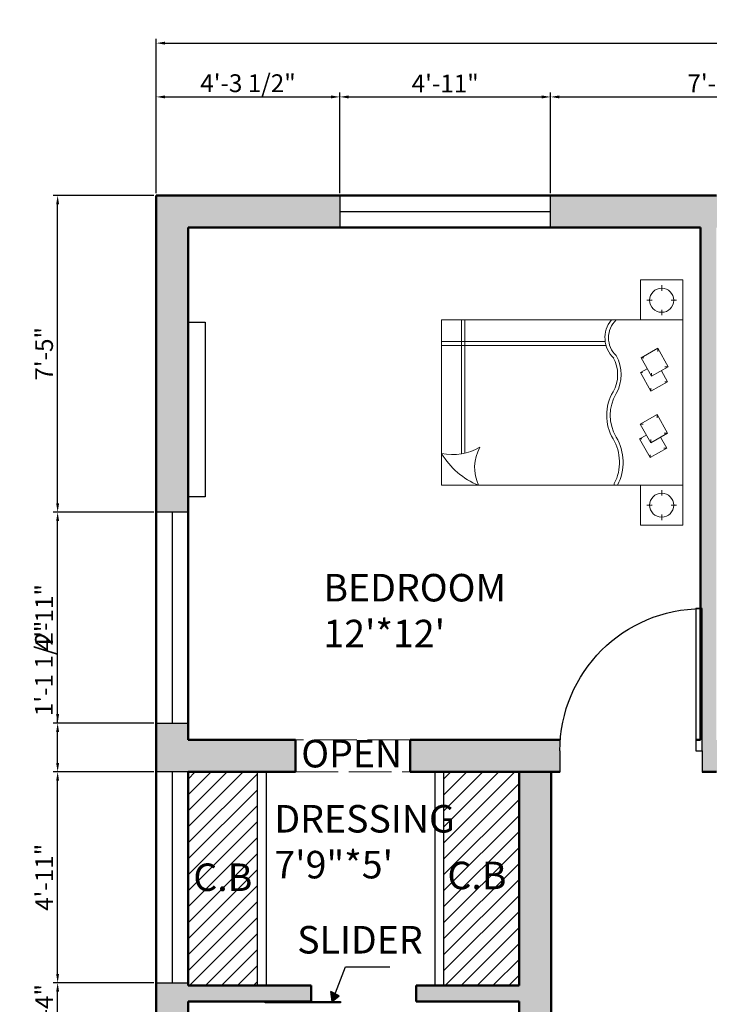
# Model space of a CAD drawing. Units: inches. Extents: x 876 to 1414, y 2665 to 3216.
# Tile 3 of 4: x 876 to 1070, y 2939 to 3216. Entities that reach past the tile are written whole.
import ezdxf

# ---------------------------------------------------------------- set-up
doc = ezdxf.new("R2010")
doc.units = ezdxf.units.IN
doc.linetypes.add('ACAD_ISO02W100', pattern=[15, 12, -3])
for name, color, linetype, lineweight in [('A-ANNO-DIMS', 2, 'Continuous', 18), ('A-ANNO-TEXT', 7, 'Continuous', 25), ('A-AREA-IDEN', 7, 'Continuous', 25), ('A-FLOR-CASE', 8, 'Continuous', 25), ('A-FLOR-CASE-PATT', 252, 'Continuous', 13), ('A-OPEN-OVHD', 210, 'ACAD_ISO02W100', 18), ('A-WALL-PATT', 252, 'Continuous', 13), ('DOOR', 52, 'Continuous', 25), ('FUR', 8, 'Continuous', 18), ('WALL', 7, 'Continuous', 50), ('WIND', 130, 'Continuous', 25)]:
    doc.layers.add(name, color=color, linetype=linetype, lineweight=lineweight)
doc.styles.get("Standard").update_dxf_attribs({"font": 'arial.ttf'})
doc.dimstyles.new('ISO-25', dxfattribs={"dimtxt": 5, "dimasz": 2.5, "dimexe": 1.25, "dimexo": 0.625, "dimtad": 1, "dimdec": 0, "dimlunit": 4, "dimtxsty": 'Standard', "dimcen": 2.5, "dimadec": 0, "dimazin": 0, "dimtfac": 1, "dimtdec": 0, "dimtmove": 0, "dimatfit": 3, "dimfxl": 1, "dimarcsym": 0})

# ---------------------------------------------------------------- blocks, each defined once
blk = doc.blocks.new('*U2')
for p, q in [((0, 0), (0, -6)), ((40, 0), (40, -6))]:
    blk.add_line(p, q)
blk.add_lwpolyline([(0, 0), (0, 40), (1.75, 40), (1.75, 0)], close=True)
blk.add_arc((0, 0), 40, 0, 90)
blk = doc.blocks.new('*D7')
at = {"layer": 'A-ANNO-DIMS', "color": 0, "lineweight": -2, "transparency": 16777216}
for p, q in [((914.52, 3167.07), (914.52, 3210.51)), ((1361.52, 3167.07), (1361.52, 3210.51)), ((917.02, 3209.26), (1359.02, 3209.26))]:
    blk.add_line(p, q, dxfattribs=at)
at = {"layer": 'A-ANNO-DIMS', "color": 0, "lineweight": 100, "transparency": 16777216}
for points in [[(917.02, 3209.68), (917.02, 3208.84), (914.52, 3209.26)], [(1359.02, 3209.68), (1359.02, 3208.84), (1361.52, 3209.26)]]:
    blk.add_solid(points, dxfattribs=at)
at = {"layer": 'Defpoints', "color": 0, "lineweight": 100, "transparency": 16777216}
for p in [(1361.52, 3209.26), (914.52, 3166.44), (1361.52, 3166.44)]:
    blk.add_point(p, dxfattribs=at)
at = {"layer": 'A-ANNO-DIMS', "color": 0, "transparency": 16777216, "insert": (1138.02, 3212.44), "char_height": 5, "attachment_point": 5}
blk.add_mtext('37\'-3"', dxfattribs=at)
blk = doc.blocks.new('BED-DOUBLE-NIGHTSTANDS')
for p, q in [((61.86, 66.59), (61.86, 67.46)), ((61.86, 66.59), (61.86, 65.9)), ((58.48, 63.21), (57.64, 63.21)), ((58.48, 63.21), (59.22, 63.21)), ((65.24, 63.21), (64.53, 63.21)), ((65.24, 63.21), (66.05, 63.21)), ((61.86, 59.83), (61.86, 60.56)), ((61.86, 59.83), (61.86, 59.02)), ((5.55, 20.02), (5.55, 57.68)), ((5.55, 20.02), (5.55, 57.68)), ((6.55, 20.22), (6.55, 57.68)), ((0, 51.64), (45.97, 51.64)), ((0, 50.51), (45.97, 50.51)), ((45.97, 50.51), (46.2, 50.51)), ((56.06, 47.08), (56.85, 47.08)), ((60.79, 49.72), (60.79, 48.79)), ((63.72, 44.49), (62.78, 44.49)), ((55.87, 42.88), (56.5, 42.88)), ((58.98, 41.84), (58.98, 42.69)), ((63.53, 40.29), (62.71, 40.29)), ((58.79, 37.65), (58.79, 38.47)), ((60.58, 31.07), (60.58, 30.14)), ((55.85, 28.43), (56.64, 28.43)), ((63.5, 25.84), (62.57, 25.84)), ((55.66, 24.23), (56.28, 24.23)), ((58.77, 23.19), (58.77, 24.04)), ((58.58, 19), (58.58, 19.82)), ((63.31, 21.64), (62.5, 21.64)), ((48.54, 11.7), (48.54, 11.24)), ((61.86, 9), (61.86, 9.87)), ((61.86, 9), (61.86, 8.3)), ((58.48, 5.62), (57.64, 5.62)), ((58.48, 5.62), (59.22, 5.62)), ((65.24, 5.62), (64.53, 5.62)), ((65.24, 5.62), (66.05, 5.62)), ((61.86, 2.24), (61.86, 2.97)), ((61.86, 2.24), (61.86, 1.43))]:
    blk.add_line(p, q)
for points in [[(67.84, 57.68), (55.89, 57.68), (55.89, 68.92), (67.84, 68.92)], [(67.84, 57.68), (0, 57.68), (0, 11.24), (67.84, 11.24)], [(60.79, 49.72), (63.72, 44.49), (58.98, 41.84), (56.06, 47.08)], [(60.58, 31.07), (63.5, 25.84), (58.77, 23.19), (55.85, 28.43)], [(67.84, 0), (55.89, 0), (55.89, 11.24), (67.84, 11.24)]]:
    blk.add_lwpolyline(points, close=True)
for points in [[(61.78, 43.41), (63.53, 40.29), (58.79, 37.65), (55.87, 42.88), (57.8, 43.96)], [(61.57, 24.76), (63.31, 21.64), (58.58, 19), (55.66, 24.23), (57.59, 25.31)]]:
    blk.add_lwpolyline(points)
for centre in [(61.86, 63.21), (61.86, 5.62)]:
    blk.add_circle(centre, 3.38)
for centre, radius, start, end in [((53.77, 52.67), 7.86, 140.4162, 226.8897), ((53.77, 52.67), 6.86, 133.1103, 226.8897), ((39.66, 42.33), 9.82, 330.4833, 29.5167), ((39.66, 42.33), 10.82, 330.4833, 29.5167), ((59.48, 30.89), 13.07, 149.6109, 210.3891), ((59.48, 30.89), 12.07, 149.6109, 210.3891), ((37, 17.69), 13, 332.5506, 30.4499), ((37, 17.69), 14, 332.5506, 30.4499), ((3.14, 34.99), 15.16, 258.0495, 300.2653), ((18.12, 30.76), 20.99, 210.3296, 248.4534), ((20.79, 16.21), 11.51, 150.3891, 205.6064)]:
    blk.add_arc(centre, radius, start, end)
blk = doc.blocks.new('*D34')
at = {"layer": 'A-ANNO-DIMS', "color": 0, "lineweight": -2, "transparency": 16777216}
for p, q in [((914.52, 3167.07), (914.52, 3195.39)), ((917.02, 3194.14), (963.64, 3194.14)), ((966.14, 3167.07), (966.14, 3195.39))]:
    blk.add_line(p, q, dxfattribs=at)
at = {"layer": 'A-ANNO-DIMS', "color": 0, "lineweight": 100, "transparency": 16777216}
for points in [[(917.02, 3194.56), (917.02, 3193.72), (914.52, 3194.14)], [(963.64, 3194.56), (963.64, 3193.72), (966.14, 3194.14)]]:
    blk.add_solid(points, dxfattribs=at)
at = {"layer": 'Defpoints', "color": 0, "lineweight": 100, "transparency": 16777216}
for p in [(966.14, 3194.14), (914.52, 3166.44), (966.14, 3166.44)]:
    blk.add_point(p, dxfattribs=at)
at = {"layer": 'A-ANNO-DIMS', "color": 0, "transparency": 16777216, "insert": (940.33, 3197.35), "char_height": 5, "attachment_point": 5}
blk.add_mtext('4\'-3 1/2"', dxfattribs=at)
blk = doc.blocks.new('*D35')
at = {"layer": 'A-ANNO-DIMS', "color": 0, "lineweight": -2, "transparency": 16777216}
for p, q in [((966.14, 3167.07), (966.14, 3195.39)), ((968.64, 3194.14), (1022.89, 3194.14)), ((1025.39, 3167.07), (1025.39, 3195.39))]:
    blk.add_line(p, q, dxfattribs=at)
at = {"layer": 'A-ANNO-DIMS', "color": 0, "lineweight": 100, "transparency": 16777216}
for points in [[(968.64, 3194.56), (968.64, 3193.72), (966.14, 3194.14)], [(1022.89, 3194.56), (1022.89, 3193.72), (1025.39, 3194.14)]]:
    blk.add_solid(points, dxfattribs=at)
at = {"layer": 'Defpoints', "color": 0, "lineweight": 100, "transparency": 16777216}
for p in [(1025.39, 3194.14), (966.14, 3166.44), (1025.39, 3166.44)]:
    blk.add_point(p, dxfattribs=at)
at = {"layer": 'A-ANNO-DIMS', "color": 0, "transparency": 16777216, "insert": (995.76, 3197.28), "char_height": 5, "attachment_point": 5}
blk.add_mtext('4\'-11"', dxfattribs=at)
blk = doc.blocks.new('*D36')
at = {"layer": 'A-ANNO-DIMS', "color": 0, "lineweight": -2, "transparency": 16777216}
for p, q in [((1025.39, 3167.07), (1025.39, 3195.39)), ((1027.89, 3194.14), (1114.91, 3194.14)), ((1117.41, 3167.07), (1117.41, 3195.39))]:
    blk.add_line(p, q, dxfattribs=at)
at = {"layer": 'A-ANNO-DIMS', "color": 0, "lineweight": 100, "transparency": 16777216}
for points in [[(1027.89, 3194.56), (1027.89, 3193.72), (1025.39, 3194.14)], [(1114.91, 3194.56), (1114.91, 3193.72), (1117.41, 3194.14)]]:
    blk.add_solid(points, dxfattribs=at)
at = {"layer": 'Defpoints', "color": 0, "lineweight": 100, "transparency": 16777216}
for p in [(1117.41, 3194.14), (1025.39, 3166.44), (1117.41, 3166.44)]:
    blk.add_point(p, dxfattribs=at)
at = {"layer": 'A-ANNO-DIMS', "color": 0, "transparency": 16777216, "insert": (1071.4, 3197.32), "char_height": 5, "attachment_point": 5}
blk.add_mtext('7\'-8"', dxfattribs=at)
blk = doc.blocks.new('*D47')
at = {"layer": 'A-ANNO-DIMS', "color": 0, "lineweight": -2, "transparency": 16777216}
for p, q in [((886.82, 3018.18), (886.82, 3046.4)), ((913.89, 3018.18), (885.57, 3018.18)), ((886.82, 3006.94), (886.82, 3015.68)), ((913.89, 3004.44), (885.57, 3004.44))]:
    blk.add_line(p, q, dxfattribs=at)
at = {"layer": 'A-ANNO-DIMS', "color": 0, "lineweight": 100, "transparency": 16777216}
for points in [[(886.4, 3015.68), (887.23, 3015.68), (886.82, 3018.18)], [(886.4, 3006.94), (887.23, 3006.94), (886.82, 3004.44)]]:
    blk.add_solid(points, dxfattribs=at)
at = {"layer": 'Defpoints', "color": 0, "lineweight": 100, "transparency": 16777216}
for p in [(886.82, 3018.18), (914.52, 3018.18), (914.52, 3004.44)]:
    blk.add_point(p, dxfattribs=at)
at = {"layer": 'A-ANNO-DIMS', "color": 0, "transparency": 16777216, "insert": (883.61, 3033.54), "char_height": 5, "attachment_point": 5, "rotation": 90}
blk.add_mtext('1\'-1 1/2"', dxfattribs=at)
blk = doc.blocks.new('*D48')
at = {"layer": 'A-ANNO-DIMS', "color": 0, "lineweight": -2, "transparency": 16777216}
for p, q in [((913.89, 3166.44), (885.57, 3166.44)), ((886.82, 3079.93), (886.82, 3163.94)), ((913.89, 3077.43), (885.57, 3077.43))]:
    blk.add_line(p, q, dxfattribs=at)
at = {"layer": 'A-ANNO-DIMS', "color": 0, "lineweight": 100, "transparency": 16777216}
for points in [[(886.4, 3163.94), (887.23, 3163.94), (886.82, 3166.44)], [(886.4, 3079.93), (887.23, 3079.93), (886.82, 3077.43)]]:
    blk.add_solid(points, dxfattribs=at)
at = {"layer": 'Defpoints', "color": 0, "lineweight": 100, "transparency": 16777216}
for p in [(886.82, 3166.44), (914.52, 3166.44), (914.52, 3077.43)]:
    blk.add_point(p, dxfattribs=at)
at = {"layer": 'A-ANNO-DIMS', "color": 0, "transparency": 16777216, "insert": (883.65, 3121.94), "char_height": 5, "attachment_point": 5, "rotation": 90}
blk.add_mtext('7\'-5"', dxfattribs=at)
blk = doc.blocks.new('*D49')
at = {"layer": 'A-ANNO-DIMS', "color": 0, "lineweight": -2, "transparency": 16777216}
for p, q in [((913.89, 3077.43), (885.57, 3077.43)), ((886.82, 3020.68), (886.82, 3074.93)), ((913.89, 3018.18), (885.57, 3018.18))]:
    blk.add_line(p, q, dxfattribs=at)
at = {"layer": 'A-ANNO-DIMS', "color": 0, "lineweight": 100, "transparency": 16777216}
for points in [[(886.4, 3074.93), (887.23, 3074.93), (886.82, 3077.43)], [(886.4, 3020.68), (887.23, 3020.68), (886.82, 3018.18)]]:
    blk.add_solid(points, dxfattribs=at)
at = {"layer": 'Defpoints', "color": 0, "lineweight": 100, "transparency": 16777216}
for p in [(886.82, 3077.43), (914.52, 3077.43), (914.52, 3018.18)]:
    blk.add_point(p, dxfattribs=at)
at = {"layer": 'A-ANNO-DIMS', "color": 0, "transparency": 16777216, "insert": (883.68, 3047.81), "char_height": 5, "attachment_point": 5, "rotation": 90}
blk.add_mtext('4\'-11"', dxfattribs=at)
blk = doc.blocks.new('*D50')
at = {"layer": 'A-ANNO-DIMS', "color": 0, "lineweight": -2, "transparency": 16777216}
for p, q in [((913.89, 3004.44), (885.57, 3004.44)), ((886.82, 2947.69), (886.82, 3001.94)), ((913.89, 2945.19), (885.57, 2945.19))]:
    blk.add_line(p, q, dxfattribs=at)
at = {"layer": 'A-ANNO-DIMS', "color": 0, "lineweight": 100, "transparency": 16777216}
for points in [[(886.4, 3001.94), (887.23, 3001.94), (886.82, 3004.44)], [(886.4, 2947.69), (887.23, 2947.69), (886.82, 2945.19)]]:
    blk.add_solid(points, dxfattribs=at)
at = {"layer": 'Defpoints', "color": 0, "lineweight": 100, "transparency": 16777216}
for p in [(886.82, 3004.44), (914.52, 3004.44), (914.52, 2945.19)]:
    blk.add_point(p, dxfattribs=at)
at = {"layer": 'A-ANNO-DIMS', "color": 0, "transparency": 16777216, "insert": (883.68, 2974.82), "char_height": 5, "attachment_point": 5, "rotation": 90}
blk.add_mtext('4\'-11"', dxfattribs=at)
blk = doc.blocks.new('*D51')
at = {"layer": 'A-ANNO-DIMS', "color": 0, "lineweight": -2, "transparency": 16777216}
for p, q in [((913.89, 2945.19), (885.57, 2945.19)), ((886.82, 2931.91), (886.82, 2942.69)), ((913.89, 2929.41), (885.57, 2929.41))]:
    blk.add_line(p, q, dxfattribs=at)
at = {"layer": 'A-ANNO-DIMS', "color": 0, "lineweight": 100, "transparency": 16777216}
for points in [[(886.4, 2942.69), (887.23, 2942.69), (886.82, 2945.19)], [(886.4, 2931.91), (887.23, 2931.91), (886.82, 2929.41)]]:
    blk.add_solid(points, dxfattribs=at)
at = {"layer": 'Defpoints', "color": 0, "lineweight": 100, "transparency": 16777216}
for p in [(886.82, 2945.19), (914.52, 2945.19), (914.52, 2929.41)]:
    blk.add_point(p, dxfattribs=at)
at = {"layer": 'A-ANNO-DIMS', "color": 0, "transparency": 16777216, "insert": (883.68, 2937.3), "char_height": 5, "attachment_point": 5, "rotation": 90}
blk.add_mtext('1\'-4"', dxfattribs=at)

msp = doc.modelspace()

# ---------------------------------------------------------------- hatches: boundary and pattern name
at = {"layer": 'A-ANNO-TEXT'}
h = msp.add_hatch(color=256, dxfattribs=at)
h.dxf.hatch_style = 1
h.paths.add_polyline_path([(965.93, 2941.55), (964.83, 2942.12), (963.99, 2939.94)])
h.paths.add_polyline_path([(964.83, 2942.12), (963.65, 2942.73), (963.99, 2939.94)])
at = {"layer": 'A-FLOR-CASE-PATT'}
h = msp.add_hatch(dxfattribs=at)
h.set_pattern_fill('ANSI31', color=256)
h.paths.add_polyline_path([(942.97, 3004.44), (923.52, 3004.44), (923.52, 2944.44), (942.97, 2944.44)])
h.paths.add_polyline_path([(1016.52, 3004.44), (995.42, 3004.44), (995.42, 2944.44), (1016.52, 2944.44)])
at = {"layer": 'A-WALL-PATT'}
h = msp.add_hatch(color=256, dxfattribs=at)
h.dxf.hatch_style = 1
h.paths.add_polyline_path([(966.14, 3166.44), (914.52, 3166.44), (914.52, 3077.43), (923.52, 3077.43), (923.52, 3157.44), (966.14, 3157.44)])
h.paths.add_polyline_path([(1117.41, 3166.44), (1072.02, 3166.44), (1025.39, 3166.44), (1025.39, 3157.44), (1067.52, 3157.44), (1067.52, 3050.33), (1068, 3050.33), (1068, 3010.33), (1068, 3004.44), (1072.02, 3004.44), (1076.39, 3004.44), (1076.39, 3010.44), (1076.39, 3013.44), (1072.02, 3013.44), (1072.02, 3157.44), (1090.31, 3157.44), (1117.41, 3157.44)])
h.paths.add_polyline_path([(1257.93, 3166.44), (1225.02, 3166.44), (1176.66, 3166.44), (1176.66, 3157.44), (1216.02, 3157.44), (1216.02, 3013.44), (1116.28, 3013.44, -0.01877), (1116.39, 3010.44), (1116.39, 3004.44), (1225.02, 3004.44), (1225.02, 3014.27), (1225.02, 3110.94), (1249.02, 3110.94), (1251.21, 3110.94), (1251.21, 3115.44), (1225.02, 3115.44), (1225.02, 3157.44), (1257.93, 3157.44)])
h.paths.add_polyline_path([(1361.52, 3166.44), (1317.18, 3166.44), (1317.18, 3157.44), (1330.83, 3157.44), (1352.52, 3157.44), (1352.52, 3115.44), (1288.77, 3115.44), (1288.77, 3110.94), (1352.52, 3110.94), (1352.52, 3103.98), (1361.52, 3103.98), (1361.52, 3115.44)])
h.paths.add_polyline_path([(1028, 3010.33, -0.01947), (1028.12, 3013.44), (985.91, 3013.44), (985.91, 3004.44), (1028, 3004.44)])
h.paths.add_polyline_path([(953.71, 3013.44), (923.52, 3013.44), (923.52, 3018.18), (914.52, 3018.18), (914.52, 3004.44), (923.52, 3004.44), (953.71, 3004.44)])
h.paths.add_polyline_path([(958.09, 2944.44), (923.52, 2944.44), (923.52, 2945.19), (914.52, 2945.19), (914.52, 2939.94), (914.52, 2929.41), (923.52, 2929.41), (923.52, 2939.94), (958.09, 2939.94)])
h.paths.add_polyline_path([(1025.52, 3004.44), (1016.52, 3004.44), (1016.52, 2944.44), (987.59, 2944.44), (987.59, 2939.94), (1016.52, 2939.94), (1016.52, 2917.71, -0.025042), (1020.12, 2917.89), (1025.52, 2917.89), (1025.52, 2939.94)])
h.paths.add_polyline_path([(923.52, 2870.94), (923.52, 2879.94), (923.52, 2896.8), (914.52, 2896.8), (914.52, 2870.94), (914.52, 2713.44), (918.61, 2713.44), (918.61, 2722.81), (923.52, 2722.81)])
h.paths.add_polyline_path([(930.9, 2722.81), (918.61, 2722.81), (918.61, 2711.51), (930.9, 2711.51)])
h.paths.add_polyline_path([(1056.58, 2722.81), (1044.28, 2722.81), (1044.28, 2711.51), (1056.58, 2711.51)])
h.paths.add_polyline_path([(1130.38, 2722.44), (1076.52, 2722.44), (1067.52, 2722.44), (1056.58, 2722.44), (1056.58, 2713.44), (1076.52, 2713.44), (1130.38, 2713.44)])
h.paths.add_polyline_path([(1213.02, 2879.94), (1142.76, 2879.94), (1142.76, 2870.94), (1208.52, 2870.94), (1208.52, 2722.44), (1213.02, 2722.44)])
h.paths.add_polyline_path([(1219.02, 2822.94), (1213.02, 2822.94), (1213.02, 2818.44), (1219.02, 2818.44)])
h.paths.add_polyline_path([(1352.52, 2822.94), (1259.02, 2822.94), (1259.02, 2818.44), (1352.52, 2818.44)])
h.paths.add_polyline_path([(1274.52, 2848.67), (1270.02, 2848.67), (1270.02, 2822.94), (1274.52, 2822.94)])
h.paths.add_polyline_path([(1352.52, 2887.44), (1270.02, 2887.44), (1270.02, 2880.56), (1274.52, 2880.56), (1274.52, 2882.94), (1352.52, 2882.94)])
h.paths.add_polyline_path([(1361.52, 2915.4), (1352.52, 2915.4), (1352.52, 2872.66), (1361.52, 2872.66)])
h.paths.add_polyline_path([(1361.52, 2840.05), (1352.52, 2840.05), (1352.52, 2722.44), (1319.37, 2722.44), (1319.37, 2713.44), (1349.52, 2713.44), (1361.52, 2713.44)])
h.paths.add_polyline_path([(1260.12, 2722.44), (1225.02, 2722.44), (1213.02, 2722.44), (1208.52, 2722.44), (1189.62, 2722.44), (1189.62, 2713.44), (1213.02, 2713.44), (1260.12, 2713.44)])
h.paths.add_polyline_path([(1361.52, 3004.44), (1361.52, 3044.73), (1352.52, 3044.73), (1352.52, 3013.44), (1352.52, 2974.65), (1361.52, 2974.65)])
h.paths.add_polyline_path([(1352.52, 3013.44), (1288.77, 3013.44), (1288.77, 3004.44), (1352.52, 3004.44)])
h.paths.add_polyline_path([(1067.52, 2845.54), (1025.52, 2845.54), (1025.52, 2870.94), (1025.52, 2881.89), (1020.12, 2881.89), (1016.52, 2881.89), (1016.52, 2879.94), (923.52, 2879.94), (923.52, 2870.94), (1016.52, 2870.94), (1016.52, 2845.54), (1016.52, 2836.54), (1025.52, 2836.54), (1067.52, 2836.54)])
h.paths.add_polyline_path([(1076.52, 2728.79), (1073.09, 2728.79), (1067.52, 2728.79), (1067.52, 2722.44), (1076.52, 2722.44)])
h.paths.add_polyline_path([(1091.93, 2866.85), (1126.41, 2866.85), (1126.41, 2882.79), (1091.93, 2882.79)], flags=9)
h.paths.add_polyline_path([(1112.49, 2839.74), (1177.4, 2839.74), (1177.4, 2868.59), (1112.49, 2868.59)], flags=9)
h.paths.add_polyline_path([(1005.34, 2789.94), (1060.41, 2789.94), (1060.41, 2818.8), (1005.34, 2818.8)], flags=9)

# ---------------------------------------------------------------- linework, layer by layer
at = {"layer": 'A-ANNO-TEXT'}
for p, q in [((963.99, 2939.94), (967.76, 2949.66)), ((967.76, 2949.66), (980.17, 2949.66)), ((963.99, 2939.94), (963.65, 2942.73)), ((963.65, 2942.73), (963.99, 2939.94)), ((965.93, 2941.55), (963.65, 2942.73)), ((963.99, 2939.94), (965.93, 2941.55))]:
    msp.add_line(p, q, dxfattribs=at)
at = {"layer": 'A-FLOR-CASE'}
for p, q in [((942.97, 2944.44), (942.97, 3004.44)), ((945.49, 2944.44), (945.49, 3004.44)), ((992.9, 2944.44), (992.9, 3004.44)), ((995.42, 2944.44), (995.42, 3004.44))]:
    msp.add_line(p, q, dxfattribs=at)
msp.add_lwpolyline([(923.52, 3130.85), (928.28, 3130.85), (928.28, 3081.75), (923.52, 3081.75)], close=True, dxfattribs=at)
at = {"layer": 'A-OPEN-OVHD'}
msp.add_lwpolyline([(953.71, 3004.44), (985.91, 3004.44), (985.91, 3013.44), (953.71, 3013.44)], close=True, dxfattribs=at)
at = {"layer": 'DOOR'}
for p, q in [((945.17, 2939.52), (945.17, 2939.94)), ((966.29, 2939.52), (945.17, 2939.52)), ((958.09, 2939.94), (966.29, 2939.94)), ((966.29, 2939.94), (966.29, 2939.52))]:
    msp.add_line(p, q, dxfattribs=at)
at = {"layer": 'WALL'}
for p, q in [((914.52, 3004.44), (914.52, 3166.44)), ((914.52, 3166.44), (1072.02, 3166.44)), ((923.52, 3157.44), (1067.52, 3157.44)), ((923.52, 3013.44), (923.52, 3157.44)), ((1067.52, 3157.44), (1067.52, 3013.44)), ((953.71, 3013.44), (923.52, 3013.44)), ((953.71, 3004.44), (953.71, 3013.44)), ((985.91, 3004.44), (985.91, 3013.44)), ((1028.12, 3013.44), (985.91, 3013.44)), ((1067.52, 3013.44), (1066.25, 3013.44)), ((914.52, 3004.44), (914.52, 2939.94)), ((923.52, 3004.44), (923.52, 2944.44)), ((953.71, 3004.44), (923.52, 3004.44)), ((1028, 3004.44), (985.91, 3004.44)), ((1016.52, 2944.44), (1016.52, 3004.44)), ((1025.52, 2939.94), (1025.52, 3004.44)), ((1072.02, 3004.44), (1068, 3004.44)), ((923.52, 2944.44), (958.09, 2944.44)), ((958.09, 2939.94), (958.09, 2944.44)), ((987.59, 2939.94), (987.59, 2944.44)), ((987.59, 2944.44), (1016.52, 2944.44)), ((914.52, 2939.94), (914.52, 2870.94)), ((923.52, 2939.94), (958.09, 2939.94)), ((923.52, 2939.94), (923.52, 2879.94)), ((987.59, 2939.94), (1016.52, 2939.94)), ((1016.52, 2917.71), (1016.52, 2939.94)), ((1025.52, 2917.89), (1025.52, 2939.94))]:
    msp.add_line(p, q, dxfattribs=at)
at = {"layer": 'WIND'}
for p, q in [((966.14, 3161.94), (1025.39, 3161.94)), ((919.02, 3077.43), (919.02, 3018.18)), ((919.02, 3004.44), (919.02, 2945.19))]:
    msp.add_line(p, q, dxfattribs=at)
for points in [[(966.14, 3157.44), (1025.39, 3157.44), (1025.39, 3166.44), (966.14, 3166.44)], [(914.52, 3077.43), (914.52, 3018.18), (923.52, 3018.18), (923.52, 3077.43)], [(914.52, 3004.44), (914.52, 2945.19), (923.52, 2945.19), (923.52, 3004.44)]]:
    msp.add_lwpolyline(points, close=True, dxfattribs=at)

# ---------------------------------------------------------------- block references
at = {"layer": 'DOOR', "xscale": -1}
msp.add_blockref('*U2', (1068, 3010.33), dxfattribs=at)
at = {"layer": 'FUR'}
msp.add_blockref('BED-DOUBLE-NIGHTSTANDS', (994.76, 3073.78), dxfattribs=at)

# ---------------------------------------------------------------- texts
at = {"layer": 'A-ANNO-TEXT', "char_height": 7.733, "attachment_point": 1}
for s, insert in [('OPEN', (955.3, 3013.44)), ('C.B', (924.96, 2978.71)), ('C.B', (996.4, 2979.21)), ('SLIDER', (954.16, 2961.14))]:
    msp.add_mtext_dynamic_manual_height_columns(s, width=254.6465, gutter_width=38.66, heights=[0], dxfattribs=dict(at, insert=insert))
at = {"layer": 'A-AREA-IDEN', "char_height": 7.733, "attachment_point": 1}
for s, insert in [("BEDROOM\\P12'*12'", (961.52, 3060.08)), ('DRESSING\\P7\'9"*5\'', (947.74, 2995.14))]:
    msp.add_mtext_dynamic_manual_height_columns(s, width=254.6465, gutter_width=38.66, heights=[0], dxfattribs=dict(at, insert=insert))

# ---------------------------------------------------------------- dimensions: what is measured, and where the dimension line sits
at = {"layer": 'A-ANNO-DIMS'}
for base, p1, p2, override, picture, middle in [((1361.52, 3209.26), (914.52, 3166.44), (1361.52, 3166.44), {"dimclrd": 0, "dimclre": 0, "dimclrt": 0}, '*D7', (1138.02, 3212.44)), ((966.14, 3194.14), (914.52, 3166.44), (966.14, 3166.44), {"dimdec": 1, "dimlfac": 1, "dimrnd": 0, "dimzin": 1, "dimdsep": 46, "dimlunit": 4, "dimfrac": 2}, '*D34', (940.33, 3197.35)), ((1025.3861, 3194.1415), (966.1373, 3166.4415), (1025.3861, 3166.4415), {"dimdec": 1, "dimlfac": 1, "dimrnd": 0, "dimzin": 1, "dimdsep": 46, "dimlunit": 4, "dimfrac": 2}, '*D35', (995.7617, 3197.2767)), ((1117.41, 3194.14), (1025.39, 3166.44), (1117.41, 3166.44), {"dimdec": 1, "dimlfac": 1, "dimrnd": 0, "dimzin": 1, "dimdsep": 46, "dimlunit": 4, "dimfrac": 2}, '*D36', (1071.4, 3197.32))]:
    dim = msp.add_linear_dim(base=base, p1=p1, p2=p2, dimstyle='ISO-25', override=override, dxfattribs=at)
    dim.commit()
    dim.dimension.update_dxf_attribs({"geometry": picture, "text_midpoint": middle})
for base, p1, p2, picture, middle in [((886.82, 3166.44), (914.52, 3077.43), (914.52, 3166.44), '*D48', (883.65, 3121.94)), ((886.8167, 3077.43), (914.5167, 3018.1812), (914.5167, 3077.43), '*D49', (883.6815, 3047.8056)), ((886.82, 3018.18), (914.52, 3004.44), (914.52, 3018.18), '*D47', (883.61, 3033.54)), ((886.8167, 3004.4415), (914.5167, 2945.1927), (914.5167, 3004.4415), '*D50', (883.6815, 2974.8171)), ((886.82, 2945.19), (914.52, 2929.41), (914.52, 2945.19), '*D51', (883.68, 2937.3))]:
    dim = msp.add_linear_dim(base=base, p1=p1, p2=p2, angle=90, dimstyle='ISO-25', override={"dimdec": 1, "dimlfac": 1, "dimrnd": 0, "dimzin": 1, "dimdsep": 46, "dimlunit": 4, "dimfrac": 2}, dxfattribs=at)
    dim.commit()
    dim.dimension.update_dxf_attribs({"geometry": picture, "text_midpoint": middle})

doc.saveas('drawing.dxf')
